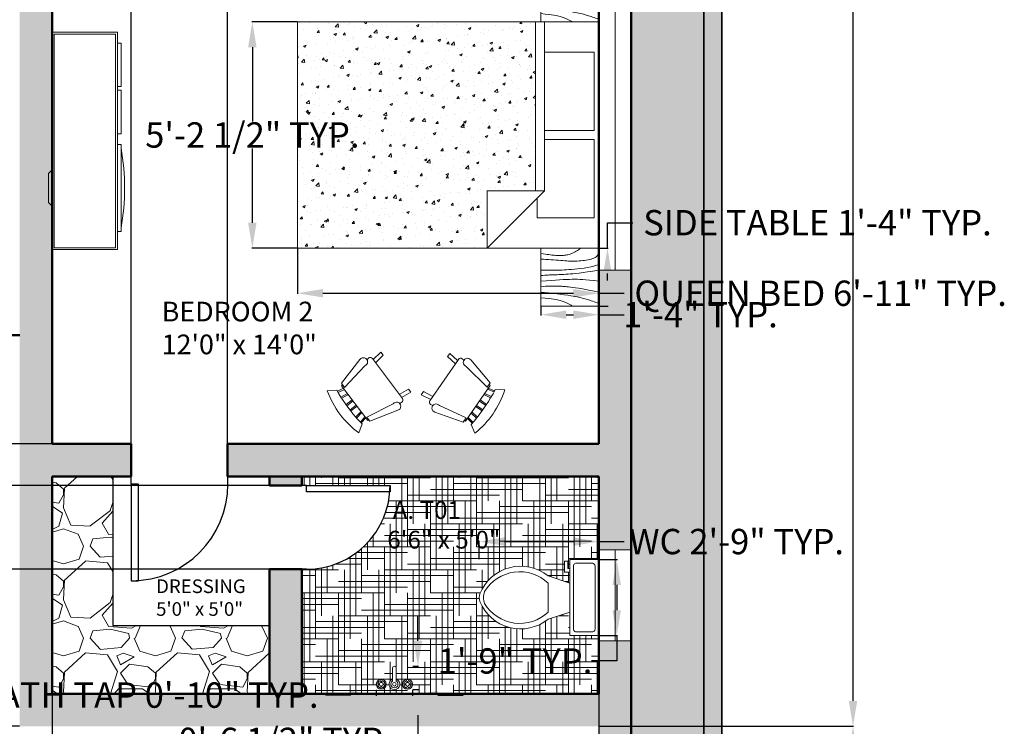
# Model space of a CAD drawing. Units: inches. Extents: x 319 to 870, y 210 to 995.
# Tile 3 of 6: x 598 to 870, y 408 to 603. Entities that reach past the tile are written whole.
import ezdxf

# ---------------------------------------------------------------- set-up
doc = ezdxf.new("R2010")
doc.units = ezdxf.units.IN
doc.header["$MEASUREMENT"] = 0
for name, color, linetype, lineweight in [('A-ANNO-DIMS', 2, 'Continuous', 18), ('A-AREA-IDEN', 7, 'Continuous', 18), ('A-DOOR', 4, 'Continuous', 25), ('A-FLOR-CASE', 7, 'Continuous', 25), ('A-FLOR-CASE-PATT', 252, 'Continuous', 13), ('A-FLOR-FIXT', 9, 'Continuous', 18), ('A-FLOR-PATT', 252, 'Continuous', 13), ('A-FURN', 8, 'Continuous', 18), ('A-GLAZ', 4, 'Continuous', 18), ('A-WALL', 7, 'Continuous', 50), ('A-WALL-PATT', 8, 'Continuous', 13), ('C-PROP', 7, 'Continuous', 35), ('C-PROP-PATT', 8, 'Continuous', 13)]:
    doc.layers.add(name, color=color, linetype=linetype, lineweight=lineweight)
doc.layers.add('A-FURN-PATT', color=30, linetype='Continuous', lineweight=13, true_color=0xf7941d)
doc.layers.add('C-SITE-PATT', color=126, linetype='Continuous', lineweight=13, true_color=0x1e6f63)
doc.styles.get("Standard").update_dxf_attribs({"font": 'arial.ttf'})
doc.dimstyles.get("Standard").update_dxf_attribs({"dimtxt": 7, "dimasz": 7, "dimexe": 0.18, "dimexo": 0.0625, "dimgap": 0.09, "dimtad": 0, "dimtih": 1, "dimtoh": 1, "dimdec": 0, "dimzin": 0, "dimdsep": 46, "dimlunit": 3, "dimtxsty": 'Standard', "dimcen": 0.09, "dimadec": 0, "dimazin": 0, "dimtfac": 1, "dimtdec": 0, "dimtofl": 0, "dimtmove": 0, "dimatfit": 3, "dimfxl": 1, "dimtolj": 1, "dimtzin": 0, "dimarcsym": 0})

# ---------------------------------------------------------------- blocks, each defined once
blk = doc.blocks.new('*U17')
for p, q in [((0, 0), (0, 6)), ((24, 0), (24, 6))]:
    blk.add_line(p, q)
blk.add_lwpolyline([(0, 0), (0, -24), (1.75, -24), (1.75, 0)], close=True)
blk.add_arc((0, 0), 24, 270, 0)
blk = doc.blocks.new('Bed - Queen')
for p, q in [((0, -80.00003), (0, 0)), ((0, 0), (59.99999, 0)), ((59.99999, 0), (59.99999, -80.00003)), ((7.99999, -1.2), (28.79998, -1.2)), ((7.99999, -14.4), (7.99999, -1.2)), ((28.79998, -1.2), (28.79998, -14.4)), ((31.19999, -1.2), (51.99999, -1.2)), ((31.19999, -14.4), (31.19999, -1.2)), ((51.99999, -1.2), (51.99999, -16.4)), ((0, -14.4), (44.8, -14.4)), ((59.99999, -29.6), (44.8, -14.4)), ((44.8, -14.4), (44.8, -29.6)), ((44.8, -16.8), (0, -16.8)), ((51.99999, -16.4), (46.79936, -16.4)), ((44.8, -29.6), (59.99999, -29.6)), ((59.99999, -80.00003), (0, -80.00003))]:
    blk.add_line(p, q)
blk = doc.blocks.new('Entertainment Center')
for p, q in [((-4, 0), (-5, -1)), ((4, 0), (-4, 0)), ((5, -1), (4, 0)), ((-17, -19), (-17, -1)), ((-17, -1), (43, -1)), ((-16.5, -18.5), (-16.5, -1.5)), ((-16.5, -1.5), (42.5, -1.5)), ((42.5, -1.5), (42.5, -18.5)), ((43, -1), (43, -19)), ((43, -19), (-17, -19)), ((42.5, -18.5), (-16.5, -18.5)), ((-12, -20), (-12, -19)), ((12, -19), (12, -20)), ((15, -20), (15, -19)), ((27, -19), (27, -20)), ((28, -20), (28, -19)), ((40, -19), (40, -20)), ((12, -20), (-12, -20)), ((27, -20), (15, -20)), ((40, -20), (28, -20))]:
    blk.add_line(p, q)
blk.add_arc((0, 40), 61, 259.6111, 280.3889)
blk = doc.blocks.new('Toilet - top')
for p, q in [((9.5, -6), (9.5, -2)), ((-8, -8.5), (-8, -8)), ((-7, -8), (-7, -9.5)), ((-4, -8), (-6, -14)), ((4, -8), (6, -14)), ((-10, -8.5), (-8, -8.5)), ((-10, -9.5), (-10, -8.5)), ((-7, -9.5), (-10, -9.5)), ((4, -14), (-4, -14))]:
    blk.add_line(p, q)
blk.add_lwpolyline([(10.5, -8), (10.5, 0), (-10.5, 0), (-10.5, -8)], close=True)
for points in [[(-9.5, -2), (-9.5, -6)], [(8.5, -1), (-8.5, -1)], [(-8.5, -7), (8.5, -7)]]:
    blk.add_lwpolyline(points)
for centre, radius, start, end in [((-8.62, -1.88), 0.884, 81.8699, 188.1301), ((8.62, -1.88), 0.884, 351.8699, 98.1301), ((-8.62, -6.12), 0.884, 171.8699, 278.1301), ((8.62, -6.12), 0.884, 261.8699, 8.1301), ((3.52, -21.58), 12.17, 141.4691, 247.9714), ((4.2, -21.82), 11.33, 136.3677, 238.9468), ((-3.52, -21.58), 12.17, 292.0284, 38.5307), ((-4.2, -21.82), 11.33, 301.053, 43.6321), ((0, -27.88), 4, 245.7318, 294.2682), ((0, -29), 4, 254.8605, 285.1395)]:
    blk.add_arc(centre, radius, start, end)
blk = doc.blocks.new('Chair - Rocking')
for p, q in [((-8, -4.5), (-10, -1.5)), ((8, -4.5), (10, -1.5)), ((-8.23428, -6.99939), (-8.3093, -7.47958)), ((-8.23041, -7), (8.23915, -7)), ((-7.5, -4.5), (-7, -7)), ((-6.5, -7), (-7.02225, -4.43)), ((-4.5, -7), (-4.96674, -4.19951)), ((-4, -7), (-4.40532, -4.16272)), ((-1.5, -4.05012), (-1.5, -7)), ((-1, -7), (-1, -4.05012)), ((1, -7), (1, -4.04655)), ((1.5, -4.05012), (1.5, -7)), ((4, -7), (4.40187, -4.18694)), ((4.5, -7), (4.96761, -4.19437)), ((6.5, -7), (7, -4.4057)), ((7.5, -4.5), (7, -7)), ((8.31071, -7.48854), (8.23449, -7.00073)), ((-9, -7.5), (-12, -18.49999)), ((-7, -7.5), (-9, -7.5)), ((-9, -18.49999), (-7, -7.5)), ((7, -7.5), (9, -7.5)), ((9, -18.49999), (7, -7.5)), ((9, -7.5), (12, -18.49999)), ((-10.36644, -20.64523), (-10.5, -21.49999)), ((10.5, -21.49999), (10.3575, -20.58798)), ((-9, -22.49999), (-9.5, -26.49999)), ((0, -22.49999), (-9.5, -22.49999)), ((-8, -26.49999), (-7.5, -22.49999)), ((0, -22.49999), (9.5, -22.49999)), ((8, -26.49999), (7.5, -22.49999)), ((9, -22.49999), (9.5, -26.49999)), ((-9.5, -26.49999), (-8, -26.49999)), ((9.5, -26.49999), (8, -26.49999))]:
    blk.add_line(p, q)
for centre, radius, start, end in [((0, -34.08333), 34.08333, 72.93847, 107.0615), ((0, -68.25004), 64.25, 93.92211, 97.15267), ((0, -68.25004), 64.25, 82.84733, 93.92211), ((-10.5, -18.99999), 1.58114, 161.5651, 18.43495), ((10.5, -18.99999), 1.58114, 161.5651, 18.43495), ((-9.5, -21.49999), 1, 180, 270), ((9.5, -21.49999), 1, 270, 0)]:
    blk.add_arc(centre, radius, start, end)
blk = doc.blocks.new('Faucet - Bathroom top')
for p, q in [((-4.107, 0.125), (-4.375, 0.125)), ((-3.75, 0.4788), (-3.75, 0.75)), ((-3.5, 0.482), (-3.5, 0.75)), ((-3.1461, 0.125), (-2.875, 0.125)), ((3.143, 0.125), (2.875, 0.125)), ((3.5, 0.4788), (3.5, 0.75)), ((3.75, 0.482), (3.75, 0.75)), ((4.1039, 0.125), (4.375, 0.125)), ((-4.1039, -0.125), (-4.375, -0.125)), ((-3.75, -0.4821), (-3.75, -0.75)), ((-3.5, -0.4789), (-3.5, -0.75)), ((-3.143, -0.125), (-2.875, -0.125)), ((-0.5, -0.8639), (-0.5, -4.5)), ((0.5, -4.5), (0.5, -0.8631)), ((3.1461, -0.125), (2.875, -0.125)), ((3.5, -0.4821), (3.5, -0.75)), ((3.75, -0.4789), (3.75, -0.75)), ((4.107, -0.125), (4.375, -0.125))]:
    blk.add_line(p, q)
for centre, radius in [((-3.625, 0), 1.375), ((-4.625, 0), 0.2795), ((-3.625, 0), 0.5), ((-3.625, 1), 0.2795), ((-2.625, 0), 0.2795), ((0, 0), 0.5), ((3.625, 0), 1.375), ((2.625, 0), 0.2795), ((3.625, 0), 0.5), ((3.625, 1), 0.2795), ((4.625, 0), 0.2795), ((-3.625, -1), 0.2795), ((3.625, -1), 0.2795)]:
    blk.add_circle(centre, radius)
for centre, radius, start, end in [((-3.625, 0), 1, 105.2407, 164.2093), ((-3.625, 0), 1, 16.44125, 74.07887), ((0, 0), 1.5, 289.6514, 250.3603), ((0, 0), 1, 300.3431, 239.7554), ((3.625, 0), 1, 106.12, 164.0884), ((3.625, 0), 1, 16.23422, 73.90469), ((-3.625, 0), 1, 196.2342, 253.9047), ((-3.625, 0), 1, 286.12, 344.0884), ((3.625, 0), 1, 196.4413, 254.0789), ((3.625, 0), 1, 285.2407, 344.2093), ((0, -4.5), 0.5, 180, 0)]:
    blk.add_arc(centre, radius, start, end)
blk = doc.blocks.new('Table - Square Woodgrain 42 x 42 in.')
blk.add_line((0, -42), (42, -42))
for points in [[(0, -4), (1.704, -4.2172), (3.2358, -4.4188), (4.615, -4.604), (5.8615, -4.7721), (6.9951, -4.9224), (8.0357, -5.0541), (9.0031, -5.1667), (9.9171, -5.2594), (10.7951, -5.3316), (11.6445, -5.3836), (12.4702, -5.4157), (13.277, -5.4283), (14.0698, -5.4217), (14.8535, -5.3964), (15.6331, -5.3526), (16.4133, -5.2908), (17.1986, -5.2103), (17.9913, -5.1062), (18.793, -4.9727), (19.6056, -4.8038), (20.4307, -4.5937), (21.2701, -4.3365), (22.1256, -4.0262), (22.9989, -3.6571), (23.888, -3.2272), (24.7756, -2.7516), (25.6408, -2.2491), (26.4624, -1.7387), (27.2195, -1.2395), (27.891, -0.7703), (28.456, -0.3501), (28.8934, 0.002)], [(0, -42), (0, 0), (42, 0), (42, -42)], [(0, -8), (1.8203, -8.1001), (3.6741, -8.2149), (5.5411, -8.3408), (7.4011, -8.4741), (9.2339, -8.6112), (11.0193, -8.7484), (12.7371, -8.8821), (14.3671, -9.0086), (15.8954, -9.1246), (17.3337, -9.2278), (18.6997, -9.3159), (20.0116, -9.387), (21.2871, -9.4389), (22.5442, -9.4696), (23.8008, -9.477), (25.0749, -9.459), (26.3791, -9.4137), (27.7049, -9.3403), (29.0383, -9.2382), (30.3655, -9.1068), (31.6728, -8.9455), (32.9461, -8.7535), (34.1717, -8.5304), (35.3358, -8.2756), (36.4268, -7.9863), (37.443, -7.6521), (38.3849, -7.2603), (39.253, -6.7986), (40.048, -6.2542), (40.7705, -5.6147), (41.421, -4.8674), (42, -4)], [(42, -12), (39.1784, -12.8621), (36.4519, -13.5654), (33.8246, -14.1294), (31.3004, -14.5731), (28.8832, -14.9161), (26.577, -15.1775), (24.3858, -15.3768), (22.3136, -15.5332), (20.3622, -15.6632), (18.5254, -15.7718), (16.7947, -15.8612), (15.1618, -15.9338), (13.6183, -15.9916), (12.1558, -16.0369), (10.7659, -16.0718), (9.4403, -16.0987), (8.1703, -16.1191), (6.9461, -16.1325), (5.7577, -16.1377), (4.595, -16.1335), (3.4479, -16.1188), (2.3064, -16.0924), (1.1604, -16.0532), (0, -16)], [(42, -16), (37.6529, -16.7365), (33.8802, -17.329), (30.6179, -17.7961), (27.8015, -18.1561), (25.3668, -18.4275), (23.2497, -18.6288), (21.3859, -18.7785), (19.7111, -18.8949), (18.1693, -18.9939), (16.7375, -19.0795), (15.401, -19.1534), (14.1449, -19.217), (12.9544, -19.2717), (11.8148, -19.3191), (10.7113, -19.3606), (9.6291, -19.3976), (8.5534, -19.4323), (7.47, -19.4689), (6.3643, -19.5122), (5.222, -19.5672), (4.0288, -19.6386), (2.7703, -19.7313), (1.4321, -19.8501), (0, -20)], [(0, -24), (3.9243, -23.6805), (7.4766, -23.4138), (10.6891, -23.1954), (13.5943, -23.0205), (16.2247, -22.8847), (18.6125, -22.7832), (20.7903, -22.7116), (22.7903, -22.6651), (24.6563, -22.642), (26.4764, -22.6507), (28.35, -22.7024), (30.3766, -22.8084), (32.6555, -22.98), (35.2861, -23.2283), (38.3678, -23.5645), (42, -24)], [(42, -32), (37.392, -31.017), (33.4585, -30.2231), (30.1291, -29.5949), (27.3334, -29.109), (25.0009, -28.742), (23.0612, -28.4707), (21.4439, -28.2716), (20.0786, -28.1215), (18.8998, -28.0002), (17.8609, -27.9014), (16.9206, -27.8219), (16.0371, -27.7588), (15.1691, -27.709), (14.2748, -27.6693), (13.3128, -27.6368), (12.2415, -27.6083), (11.0295, -27.5824), (9.6867, -27.5643), (8.233, -27.5608), (6.6884, -27.5787), (5.0728, -27.6248), (3.4062, -27.7058), (1.7086, -27.8286), (0, -28)], [(0, -32), (5.4026, -32.5358), (9.9494, -33.019), (13.7424, -33.4553), (16.8834, -33.8505), (19.4743, -34.2106), (21.6171, -34.5413), (23.4136, -34.8486), (24.9657, -35.1382), (26.3614, -35.4156), (27.6332, -35.6841), (28.7995, -35.9467), (29.8788, -36.2064), (30.8897, -36.4661), (31.8507, -36.7288), (32.7802, -36.9973), (33.6968, -37.2747), (34.6175, -37.5635), (35.5531, -37.8651), (36.5128, -38.1805), (37.506, -38.5108), (38.5421, -38.8568), (39.6302, -39.2197), (40.7797, -39.6004), (42, -40)], [(0, -36), (3.0098, -36.2857), (5.5354, -36.5643), (7.6368, -36.8359), (9.374, -37.1009), (10.807, -37.3597), (11.9957, -37.6126), (13.0002, -37.8599), (13.8804, -38.102), (14.6874, -38.3393), (15.4365, -38.5729), (16.1338, -38.8041), (16.7858, -39.0341), (17.3987, -39.264), (17.9787, -39.4952), (18.5322, -39.7288), (19.0655, -39.9662), (19.5832, -40.2081), (20.0842, -40.4544), (20.5657, -40.7046), (21.0249, -40.9581), (21.459, -41.2144), (21.8653, -41.4731), (22.2409, -41.7335), (22.5831, -41.9951)]]:
    blk.add_lwpolyline(points)
blk = doc.blocks.new('*U19')
for p, q in [((0, 0), (0, -6)), ((24, 0), (24, -6))]:
    blk.add_line(p, q)
blk.add_lwpolyline([(0, 0), (0, 24), (1.75, 24), (1.75, 0)], close=True)
blk.add_arc((0, 0), 24, 0, 90)
blk = doc.blocks.new('*D27')
at = {"layer": 'A-ANNO-DIMS', "color": 0, "lineweight": -2, "transparency": 16777216}
for p, q in [((760.08, 539.7), (760.08, 546.7)), ((760.08, 546.7), (767.08, 546.7)), ((757.75, 539.7), (760.26, 539.7)), ((760.08, 530.7), (760.08, 532.7)), ((757.75, 523.7), (760.26, 523.7))]:
    blk.add_line(p, q, dxfattribs=at)
at = {"layer": 'A-ANNO-DIMS', "color": 0, "transparency": 16777216}
for points in [[(758.92, 532.7), (761.25, 532.7), (760.08, 539.7)], [(758.92, 530.7), (761.25, 530.7), (760.08, 523.7)]]:
    blk.add_solid(points, dxfattribs=at)
at = {"layer": 'Defpoints', "color": 0, "transparency": 16777216}
for p in [(757.68, 539.7), (760.08, 539.7), (757.68, 523.7)]:
    blk.add_point(p, dxfattribs=at)
at = {"layer": 'A-ANNO-DIMS', "color": 0, "transparency": 16777216, "insert": (818.11, 546.7), "char_height": 7, "attachment_point": 5}
blk.add_mtext('\\A1;SIDE TABLE 1\'-4" TYP.', dxfattribs=at)
blk = doc.blocks.new('*D28')
at = {"layer": 'A-ANNO-DIMS', "color": 0, "lineweight": -2, "transparency": 16777216}
for p, q in [((741.69, 523.64), (741.69, 521.12)), ((757.68, 523.64), (757.68, 521.12)), ((748.69, 521.3), (750.68, 521.3)), ((757.68, 521.3), (764.68, 521.3))]:
    blk.add_line(p, q, dxfattribs=at)
at = {"layer": 'A-ANNO-DIMS', "color": 0, "transparency": 16777216}
for points in [[(748.69, 522.47), (748.69, 520.14), (741.69, 521.3)], [(750.68, 522.47), (750.68, 520.14), (757.68, 521.3)]]:
    blk.add_solid(points, dxfattribs=at)
at = {"layer": 'Defpoints', "color": 0, "transparency": 16777216}
for p in [(741.69, 523.7), (757.68, 523.7), (757.68, 521.3)]:
    blk.add_point(p, dxfattribs=at)
at = {"layer": 'A-ANNO-DIMS', "color": 0, "transparency": 16777216, "insert": (785.78, 521.3), "char_height": 7, "attachment_point": 5}
blk.add_mtext('\\A1;1\'-4" TYP.', dxfattribs=at)
blk = doc.blocks.new('*D31')
at = {"layer": 'A-ANNO-DIMS', "color": 0, "lineweight": -2, "transparency": 16777216}
for p, q in [((674.45, 539.64), (674.45, 527.04)), ((757.68, 539.64), (757.68, 527.04)), ((681.45, 527.22), (750.68, 527.22)), ((757.68, 527.22), (764.68, 527.22))]:
    blk.add_line(p, q, dxfattribs=at)
at = {"layer": 'A-ANNO-DIMS', "color": 0, "transparency": 16777216}
for points in [[(681.45, 528.39), (681.45, 526.05), (674.45, 527.22)], [(750.68, 528.39), (750.68, 526.05), (757.68, 527.22)]]:
    blk.add_solid(points, dxfattribs=at)
at = {"layer": 'Defpoints', "color": 0, "transparency": 16777216}
for p in [(674.45, 539.7), (757.68, 539.7), (757.68, 527.22)]:
    blk.add_point(p, dxfattribs=at)
at = {"layer": 'A-ANNO-DIMS', "color": 0, "transparency": 16777216, "insert": (818.98, 527.22), "char_height": 7, "attachment_point": 5}
blk.add_mtext('\\A1;QUEEN BED 6\'-11" TYP.', dxfattribs=at)
blk = doc.blocks.new('*D32')
at = {"layer": 'A-ANNO-DIMS', "color": 0, "lineweight": -2, "transparency": 16777216}
for p, q in [((674.39, 602.13), (661.79, 602.13)), ((661.97, 595.13), (661.97, 574.63)), ((661.97, 546.7), (661.97, 567.21)), ((674.39, 539.7), (661.79, 539.7))]:
    blk.add_line(p, q, dxfattribs=at)
at = {"layer": 'A-ANNO-DIMS', "color": 0, "transparency": 16777216}
for points in [[(660.8, 595.13), (663.13, 595.13), (661.97, 602.13)], [(660.8, 546.7), (663.13, 546.7), (661.97, 539.7)]]:
    blk.add_solid(points, dxfattribs=at)
at = {"layer": 'Defpoints', "color": 0, "transparency": 16777216}
for p in [(674.45, 602.13), (661.97, 539.7), (674.45, 539.7)]:
    blk.add_point(p, dxfattribs=at)
at = {"layer": 'A-ANNO-DIMS', "color": 0, "transparency": 16777216, "insert": (661.97, 570.92), "char_height": 7, "attachment_point": 5}
blk.add_mtext('\\A1;5\'-2 1/2" TYP.', dxfattribs=at)
blk = doc.blocks.new('*D35')
at = {"layer": 'A-ANNO-DIMS', "color": 0, "lineweight": -2, "transparency": 16777216}
for p, q in [((654.78, 626.45), (654.78, 610.9)), ((757.68, 626.45), (757.68, 610.9)), ((661.78, 611.08), (666.54, 611.08)), ((750.68, 611.08), (745.92, 611.08))]:
    blk.add_line(p, q, dxfattribs=at)
at = {"layer": 'A-ANNO-DIMS', "color": 0, "transparency": 16777216}
for points in [[(661.78, 612.24), (661.78, 609.91), (654.78, 611.08)], [(750.68, 612.24), (750.68, 609.91), (757.68, 611.08)]]:
    blk.add_solid(points, dxfattribs=at)
at = {"layer": 'Defpoints', "color": 0, "transparency": 16777216}
for p in [(654.78, 626.51), (757.68, 626.51), (757.68, 611.08)]:
    blk.add_point(p, dxfattribs=at)
at = {"layer": 'A-ANNO-DIMS', "color": 0, "transparency": 16777216, "insert": (706.23, 611.08), "char_height": 7, "attachment_point": 5}
blk.add_mtext('\\A1;WARDROBE 8\'-7"', dxfattribs=at)
blk = doc.blocks.new('*D37')
at = {"layer": 'A-ANNO-DIMS', "color": 0, "lineweight": -2, "transparency": 16777216}
for p, q in [((724.64, 453.77), (724.64, 458.85)), ((731.64, 458.67), (750.68, 458.67)), ((757.68, 453.77), (757.68, 458.85)), ((757.68, 458.67), (764.68, 458.67))]:
    blk.add_line(p, q, dxfattribs=at)
at = {"layer": 'A-ANNO-DIMS', "color": 0, "transparency": 16777216}
for points in [[(731.64, 459.83), (731.64, 457.5), (724.64, 458.67)], [(750.68, 459.83), (750.68, 457.5), (757.68, 458.67)]]:
    blk.add_solid(points, dxfattribs=at)
at = {"layer": 'Defpoints', "color": 0, "transparency": 16777216}
for p in [(757.68, 458.67), (724.64, 453.71), (757.68, 453.71)]:
    blk.add_point(p, dxfattribs=at)
at = {"layer": 'A-ANNO-DIMS', "color": 0, "transparency": 16777216, "insert": (795.76, 458.67), "char_height": 7, "attachment_point": 5}
blk.add_mtext('\\A1;WC 2\'-9" TYP.', dxfattribs=at)
blk = doc.blocks.new('*D38')
at = {"layer": 'A-ANNO-DIMS', "color": 0, "lineweight": -2, "transparency": 16777216}
for p, q in [((757.75, 453.71), (762.82, 453.71)), ((762.64, 446.71), (762.64, 439.71)), ((757.75, 432.71), (762.82, 432.71)), ((762.64, 432.71), (762.64, 425.71)), ((762.64, 425.71), (755.64, 425.71))]:
    blk.add_line(p, q, dxfattribs=at)
at = {"layer": 'A-ANNO-DIMS', "color": 0, "transparency": 16777216}
for points in [[(761.48, 446.71), (763.81, 446.71), (762.64, 453.71)], [(761.48, 439.71), (763.81, 439.71), (762.64, 432.71)]]:
    blk.add_solid(points, dxfattribs=at)
at = {"layer": 'Defpoints', "color": 0, "transparency": 16777216}
for p in [(757.68, 453.71), (757.68, 432.71), (762.64, 432.71)]:
    blk.add_point(p, dxfattribs=at)
at = {"layer": 'A-ANNO-DIMS', "color": 0, "transparency": 16777216, "insert": (734.55, 425.71), "char_height": 7, "attachment_point": 5}
blk.add_mtext('\\A1;1\'-9" TYP.', dxfattribs=at)
blk = doc.blocks.new('*D39')
at = {"layer": 'A-ANNO-DIMS', "color": 0, "lineweight": -2, "transparency": 16777216}
for p, q in [((689.21, 416.28), (682.21, 416.28)), ((696.21, 417.72), (696.21, 416.1)), ((706.21, 417.72), (706.21, 416.1)), ((713.21, 416.28), (720.21, 416.28))]:
    blk.add_line(p, q, dxfattribs=at)
at = {"layer": 'A-ANNO-DIMS', "color": 0, "transparency": 16777216}
for points in [[(689.21, 417.45), (689.21, 415.11), (696.21, 416.28)], [(713.21, 417.45), (713.21, 415.11), (706.21, 416.28)]]:
    blk.add_solid(points, dxfattribs=at)
at = {"layer": 'Defpoints', "color": 0, "transparency": 16777216}
for p in [(696.21, 417.78), (696.21, 416.28), (706.21, 417.78)]:
    blk.add_point(p, dxfattribs=at)
at = {"layer": 'A-ANNO-DIMS', "color": 0, "transparency": 16777216, "insert": (632.95, 416.28), "char_height": 7, "attachment_point": 5}
blk.add_mtext('\\A1;BATH TAP 0\'-10" TYP.', dxfattribs=at)
blk = doc.blocks.new('*D40')
at = {"layer": 'A-ANNO-DIMS', "color": 0, "lineweight": -2, "transparency": 16777216}
for p, q in [((707.71, 431.28), (707.71, 438.28)), ((706.27, 424.28), (707.89, 424.28)), ((706.27, 417.78), (707.89, 417.78)), ((707.71, 410.78), (707.71, 403.78)), ((707.71, 403.78), (700.71, 403.78))]:
    blk.add_line(p, q, dxfattribs=at)
at = {"layer": 'A-ANNO-DIMS', "color": 0, "transparency": 16777216}
for points in [[(706.54, 431.28), (708.87, 431.28), (707.71, 424.28)], [(706.54, 410.78), (708.87, 410.78), (707.71, 417.78)]]:
    blk.add_solid(points, dxfattribs=at)
at = {"layer": 'Defpoints', "color": 0, "transparency": 16777216}
for p in [(706.21, 424.28), (706.21, 417.78), (707.71, 417.78)]:
    blk.add_point(p, dxfattribs=at)
at = {"layer": 'A-ANNO-DIMS', "color": 0, "transparency": 16777216, "insert": (671.13, 403.78), "char_height": 7, "attachment_point": 5}
blk.add_mtext('\\A1;0\'-6 1/2" TYP.', dxfattribs=at)
blk = doc.blocks.new('*D50')
at = {"layer": 'A-ANNO-DIMS', "color": 0, "lineweight": -2, "transparency": 16777216}
for p, q in [((766.75, 923.67), (828.11, 923.67)), ((827.93, 916.67), (827.93, 669.33)), ((827.93, 414.67), (827.93, 662)), ((757.75, 407.67), (828.11, 407.67))]:
    blk.add_line(p, q, dxfattribs=at)
at = {"layer": 'A-ANNO-DIMS', "color": 0, "transparency": 16777216}
for points in [[(826.77, 916.67), (829.1, 916.67), (827.93, 923.67)], [(826.77, 414.67), (829.1, 414.67), (827.93, 407.67)]]:
    blk.add_solid(points, dxfattribs=at)
at = {"layer": 'Defpoints', "color": 0, "transparency": 16777216}
for p in [(766.68, 923.67), (827.93, 923.67), (757.68, 407.67)]:
    blk.add_point(p, dxfattribs=at)
at = {"layer": 'A-ANNO-DIMS', "color": 0, "transparency": 16777216, "insert": (827.93, 665.67), "char_height": 7, "attachment_point": 5}
blk.add_mtext('\\A1;43\'-0"', dxfattribs=at)
blk = doc.blocks.new('*D51')
at = {"layer": 'A-ANNO-DIMS', "color": 0, "lineweight": -2, "transparency": 16777216}
for p, q in [((757.75, 407.67), (828.11, 407.67)), ((827.93, 400.67), (827.93, 369.83)), ((827.93, 331.67), (827.93, 362.5)), ((791.75, 324.67), (828.11, 324.67))]:
    blk.add_line(p, q, dxfattribs=at)
at = {"layer": 'A-ANNO-DIMS', "color": 0, "transparency": 16777216}
for points in [[(826.77, 400.67), (829.1, 400.67), (827.93, 407.67)], [(826.77, 331.67), (829.1, 331.67), (827.93, 324.67)]]:
    blk.add_solid(points, dxfattribs=at)
at = {"layer": 'Defpoints', "color": 0, "transparency": 16777216}
for p in [(757.68, 407.67), (827.93, 407.67), (791.68, 324.67)]:
    blk.add_point(p, dxfattribs=at)
at = {"layer": 'A-ANNO-DIMS', "color": 0, "transparency": 16777216, "insert": (827.93, 366.17), "char_height": 7, "attachment_point": 5}
blk.add_mtext('\\A1;6\'-11"', dxfattribs=at)
blk = doc.blocks.new('*D53')
at = {"layer": 'A-ANNO-DIMS', "color": 0, "lineweight": -2, "transparency": 16777216}
for p, q in [((606.68, 416.61), (606.68, 214.45)), ((757.68, 416.61), (757.68, 214.45)), ((613.68, 214.63), (670.4, 214.63)), ((750.68, 214.63), (693.97, 214.63))]:
    blk.add_line(p, q, dxfattribs=at)
at = {"layer": 'A-ANNO-DIMS', "color": 0, "transparency": 16777216}
for points in [[(613.68, 215.8), (613.68, 213.47), (606.68, 214.63)], [(750.68, 215.8), (750.68, 213.47), (757.68, 214.63)]]:
    blk.add_solid(points, dxfattribs=at)
at = {"layer": 'Defpoints', "color": 0, "transparency": 16777216}
for p in [(606.68, 416.67), (757.68, 416.67), (757.68, 214.63)]:
    blk.add_point(p, dxfattribs=at)
at = {"layer": 'A-ANNO-DIMS', "color": 0, "transparency": 16777216, "insert": (682.18, 214.63), "char_height": 7, "attachment_point": 5}
blk.add_mtext('\\A1;12\'-7"', dxfattribs=at)
blk = doc.blocks.new('*D54')
at = {"layer": 'A-ANNO-DIMS', "color": 0, "lineweight": -2, "transparency": 16777216}
for p, q in [((606.62, 485.67), (334.2, 485.67)), ((334.38, 478.67), (334.38, 450.33)), ((334.38, 414.67), (334.38, 443)), ((597.62, 407.67), (334.2, 407.67))]:
    blk.add_line(p, q, dxfattribs=at)
at = {"layer": 'A-ANNO-DIMS', "color": 0, "transparency": 16777216}
for points in [[(333.21, 478.67), (335.55, 478.67), (334.38, 485.67)], [(333.21, 414.67), (335.55, 414.67), (334.38, 407.67)]]:
    blk.add_solid(points, dxfattribs=at)
at = {"layer": 'Defpoints', "color": 0, "transparency": 16777216}
for p in [(334.38, 485.67), (606.68, 485.67), (597.68, 407.67)]:
    blk.add_point(p, dxfattribs=at)
at = {"layer": 'A-ANNO-DIMS', "color": 0, "transparency": 16777216, "insert": (334.38, 446.67), "char_height": 7, "attachment_point": 5}
blk.add_mtext('\\A1;6\'-6"', dxfattribs=at)
blk = doc.blocks.new('*D55')
at = {"layer": 'A-ANNO-DIMS', "color": 0, "lineweight": -2, "transparency": 16777216}
for p, q in [((628.53, 485.73), (628.53, 985.1)), ((635.53, 984.92), (648.14, 984.92)), ((655.14, 485.73), (655.14, 985.1)), ((655.14, 984.92), (662.14, 984.92))]:
    blk.add_line(p, q, dxfattribs=at)
at = {"layer": 'A-ANNO-DIMS', "color": 0, "transparency": 16777216}
for points in [[(635.53, 986.09), (635.53, 983.75), (628.53, 984.92)], [(648.14, 986.09), (648.14, 983.75), (655.14, 984.92)]]:
    blk.add_solid(points, dxfattribs=at)
at = {"layer": 'Defpoints', "color": 0, "transparency": 16777216}
for p in [(655.14, 984.92), (628.53, 485.67), (655.14, 485.67)]:
    blk.add_point(p, dxfattribs=at)
at = {"layer": 'A-ANNO-DIMS', "color": 0, "transparency": 16777216, "insert": (679.75, 984.92), "char_height": 7, "attachment_point": 5}
blk.add_mtext('\\A1;2\'-2 1/2"', dxfattribs=at)
blk = doc.blocks.new('*D56')
at = {"layer": 'A-ANNO-DIMS', "color": 0, "lineweight": -2, "transparency": 16777216}
for p, q in [((675.62, 474.1), (334.2, 474.1)), ((334.38, 467.1), (334.38, 466.2)), ((334.38, 458.09), (334.38, 458.99)), ((675.62, 451.09), (334.2, 451.09))]:
    blk.add_line(p, q, dxfattribs=at)
at = {"layer": 'A-ANNO-DIMS', "color": 0, "transparency": 16777216}
for points in [[(333.21, 467.1), (335.55, 467.1), (334.38, 474.1)], [(333.21, 458.09), (335.55, 458.09), (334.38, 451.09)]]:
    blk.add_solid(points, dxfattribs=at)
at = {"layer": 'Defpoints', "color": 0, "transparency": 16777216}
for p in [(334.38, 474.1), (675.68, 474.1), (675.68, 451.09)]:
    blk.add_point(p, dxfattribs=at)
at = {"layer": 'A-ANNO-DIMS', "color": 0, "transparency": 16777216, "insert": (334.38, 462.6), "char_height": 7, "attachment_point": 5}
blk.add_mtext('\\A1;1\'-11"', dxfattribs=at)

msp = doc.modelspace()

# ---------------------------------------------------------------- hatches: boundary and pattern name
at = {"layer": 'A-FLOR-CASE-PATT'}
h = msp.add_hatch(dxfattribs=at)
h.set_pattern_fill('GRAVEL', color=256)
h.set_pattern_definition([(228.0128, (18.288, 25.4), (-203.2, -228.6), [3.4172, -338.30484]), (184.96974, (16.002, 22.86), (304.7999999, 25.4000014), [5.86405, -580.5405]), (132.51045, (10.16, 22.352), (254, -279.4), [4.1348, -409.34723]), (267.27369, (0.254, 16.002), (25.4, 508), [5.34005, -528.66437]), (292.83365, (0, 10.668), (-127, 304.8), [5.23634, -518.3981]), (357.27369, (2.032, 5.842), (-508, 25.4), [5.34005, -528.66437]), (37.69424, (7.366, 5.588), (-330.2, -254), [7.06194, -699.13115]), (72.25533, (12.954, 9.906), (177.8, 558.8), [6.6672, -660.05257]), (121.42957, (14.986, 16.256), (-203.2, 330.2), [5.35813, -530.45546]), (175.23636, (12.192, 20.828), (279.4, -25.4), [6.11713, -299.73937]), (222.39744, (6.096, 21.336), (-304.8, -279.4), [7.91078, -783.16773]), (138.81407, (25.4, 15.748), (-177.8, 152.4), [2.70005, -267.30566]), (171.46923, (23.368, 17.526), (330.2, -50.8), [5.1368, -508.5464]), (225, (18.288, 18.288), (-4e-15, -25.4), [3.5921, -32.3289]), (203.1986, (16.51, 21.336), (127, 50.8), [1.9344, -191.5062]), (291.8014, (14.732, 20.574), (-25.4, 76.2), [2.73566, -134.0475]), (30.96376, (15.748, 18.034), (76.2, 50.8), [4.4432, -143.663]), (161.565, (19.558, 20.32), (50.8, -25.4), [3.2129, -77.109]), (16.38954, (0, 20.574), (254, 76.2), [4.5009, -445.58827]), (70.34618, (4.318, 21.844), (-101.6, -279.4), [3.776, -373.82216]), (293.1986, (19.558, 25.4), (-50.8, 127), [3.8688, -189.57184]), (343.61046, (21.082, 21.844), (-254, 76.2), [4.5009, -445.58827]), (339.44395, (0, 4.826), (-127, 50.8), [4.34035, -212.67734]), (294.77514, (4.064, 3.302), (-127, 279.4), [3.6367, -360.03593]), (66.8014, (19.812, 0), (50.8, 127), [3.8688, -189.57184]), (17.35402, (21.336, 3.556), (-330.2, -101.6), [4.25783, -421.52376]), (69.44395, (7.366, 0), (-50.8, -127), [2.1702, -214.8475]), (101.3099, (18.288, 0), (-25.4, 101.6), [1.29515, -128.21995]), (165.9638, (18.034, 1.27), (76.2, -25.4), [5.23634, -99.49055]), (186.009, (12.954, 2.54), (254, 25.4), [4.85267, -480.41365]), (303.6901, (15.748, 15.748), (-25.4, 50.8), [3.66324, -87.91776]), (353.15723, (17.78, 12.7), (431.8, -50.8), [6.39557, -633.1601]), (60.9454, (24.13, 11.938), (-101.6, -177.8), [2.6151, -258.8939]), (90, (25.4, 14.224), (-25.4, 25.4), [1.524, -23.876]), (120.25644, (12.446, 3.302), (101.6, -177.8), [3.52867, -349.3394]), (48.0128, (10.668, 6.35), (203.2, 228.6), [6.83443, -334.8876]), (0, (15.24, 11.43), (25.4, 25.4), [6.604, -18.796]), (325.30485, (21.844, 11.43), (254, -177.8), [4.0161, -397.59317]), (254.0546, (25.146, 9.144), (-25.4, -101.6), [3.6983, -181.2165]), (207.64598, (24.13, 5.588), (-482.6, -254), [6.02145, -596.12464]), (175.42608, (18.796, 2.794), (-330.2, 25.4), [6.3703, -630.65846])])
h.paths.add_polyline_path([(623.41, 476.67), (606.68, 476.67), (606.68, 416.67), (666.68, 416.67), (666.68, 435.49), (623.41, 435.49)])
at = {"layer": 'A-FLOR-PATT'}
h = msp.add_hatch(dxfattribs=at)
h.set_pattern_fill('HOUND', color=256)
h.set_pattern_definition([(0, (0, 0), (6.35, 1.5875), [25.4, -12.7]), (90, (0, 0), (-1.5875, -6.35), [25.4, -12.7])])
h.paths.add_polyline_path([(757.68, 416.67), (757.68, 432.71), (749.68, 432.71), (749.68, 439.21), (743.69, 437.21, -0.501323), (724.82, 442.16, -0.132891), (724.82, 444.25, -0.501317), (743.68, 449.21), (749.68, 447.21), (749.68, 450.21), (748.18, 450.21), (748.18, 453.21), (749.18, 453.21), (749.18, 451.21), (749.68, 451.21), (749.68, 453.71), (757.68, 453.71), (757.68, 476.67), (675.68, 476.67), (675.68, 474.1), (676.95, 474.1), (700.01, 474.1), (700.01, 472.42), (699.95, 472.42, -0.392996), (676.95, 451.04), (675.68, 451.04), (675.68, 416.67)])
h.paths.add_polyline_path([(701.71, 423.78), (701.71, 420.69, -5.828427), (700.71, 420.69), (700.71, 423.78, -1)], flags=16)
h.paths.add_polyline_path([(706.11, 419.28, -0.455903), (705.79, 419, -0.257992), (705.11, 418.32, -0.61268), (704.83, 417.9, 0.394698)], flags=16)
h.paths.add_polyline_path([(704.96, 420.03), (704.96, 419.76, -0.414214), (705.32, 419.15), (705.31, 419.15), (705.31, 419.42, -1.020482), (704.35, 419.15), (704.08, 419.15, -1.951411), (703.87, 419.56, -0.257992), (704.55, 420.24, -1.951411)], flags=16)
h.paths.add_polyline_path([(701.71, 419.28, -1), (700.71, 419.28, -1)], flags=0)
h.paths.add_polyline_path([(698.86, 419.28, -0.455903), (698.54, 419, -0.257992), (697.86, 418.32, -0.61268), (697.58, 417.9, 0.394698)], flags=16)
h.paths.add_polyline_path([(697.71, 420.03), (697.71, 419.76, -0.414214), (698.07, 419.15), (698.06, 419.15), (698.06, 419.42, -1.020482), (697.1, 419.15), (696.83, 419.15, -1.951411), (696.62, 419.56, -0.257992), (697.3, 420.24, -1.951411)], flags=16)
h.paths.add_polyline_path([(697.76, 454.02), (730.18, 454.02), (730.18, 472.33), (697.76, 472.33)], flags=24)
at = {"layer": 'A-FURN-PATT'}
h = msp.add_hatch(dxfattribs=at)
h.set_pattern_fill('AR-CONC', color=256)
h.set_pattern_definition([(50, (0, 0), (7.172602, -0.62752), [0.75, -8.25]), (355, (0, 0), (-1.387513, 7.52192), [0.6, -6.6]), (100.45144, (0.598, -0.052), (5.78509, 6.8944), [0.6374, -7.01142]), (46.1842, (0, 2), (10.67241, -1.65519), [1.125, -12.375]), (96.6356, (0.889, 1.862), (9.34662, 9.74119), [0.9561, -10.51714]), (351.1842, (0, 2), (9.34662, 9.74119), [0.9, -9.9]), (21, (1, 1.5), (5.96907, -4.02619), [0.75, -8.25]), (326, (1, 1.5), (2.433153, 7.2515), [0.6, -6.6]), (71.45144, (1.4974, 1.1645), (8.402224, 3.22531), [0.6374, -7.01142]), (37.5, (0, 0), (0.1215986, 3.3289385), [0, -6.52, 0, -6.7, 0, -6.625]), (7.5, (0, 0), (2.630695, 3.944117), [0, -3.82, 0, -6.37, 0, -2.525]), (327.5, (-2.23, 0), (5.338224, -0.225549), [0, -2.5, 0, -7.8, 0, -10.35]), (317.5, (-3.23, 0), (5.831862, 1.00105), [0, -3.25, 0, -5.18, 0, -7.35])])
h.paths.add_polyline_path([(726.89, 555.52), (740.21, 555.52), (740.21, 602.13), (674.45, 602.13), (674.45, 539.7), (726.89, 539.7)])
at = {"layer": 'A-WALL-PATT'}
h = msp.add_hatch(color=256, dxfattribs=at)
h.dxf.hatch_style = 1
h.paths.add_polyline_path([(606.68, 476.67), (628.53, 476.67), (628.53, 485.67), (606.68, 485.67), (606.68, 614.99), (597.68, 614.99), (597.68, 407.67), (757.68, 407.67), (757.68, 385.48), (766.68, 385.48), (766.68, 431.25), (757.68, 431.25), (757.68, 416.67), (606.68, 416.67)])
h = msp.add_hatch(color=256, dxfattribs=at)
h.dxf.hatch_style = 1
h.paths.add_polyline_path([(757.68, 485.67), (655.14, 485.67), (655.14, 476.67), (757.68, 476.67), (757.68, 456.34), (766.68, 456.34), (766.68, 533.56), (757.68, 533.56)])
h = msp.add_hatch(color=256, dxfattribs=at)
h.dxf.hatch_style = 1
h.paths.add_polyline_path([(675.68, 474.1), (675.68, 476.67), (666.68, 476.67), (666.68, 474.1)])
h = msp.add_hatch(color=256, dxfattribs=at)
h.dxf.hatch_style = 1
h.paths.add_polyline_path([(675.68, 451.09), (666.68, 451.09), (666.68, 416.67), (675.68, 416.67)])
at = {"layer": 'C-PROP-PATT'}
h = msp.add_hatch(color=256, dxfattribs=at)
h.dxf.hatch_style = 1
h.paths.add_polyline_path([(757.68, 329.67), (597.68, 329.67), (597.68, 324.67), (791.68, 324.67), (791.68, 948.67), (376.68, 948.67), (376.68, 943.67), (786.68, 943.67), (786.68, 329.67), (766.68, 329.67), (766.68, 354.04), (757.68, 354.04)])
at = {"layer": 'C-SITE-PATT'}
h = msp.add_hatch(color=256, dxfattribs=at)
h.dxf.hatch_style = 1
h.paths.add_polyline_path([(376.68, 515.67), (396.68, 515.67), (396.68, 923.67), (528.68, 923.67), (606.68, 923.67), (766.68, 923.67), (766.68, 329.67), (786.68, 329.67), (786.68, 943.67), (376.68, 943.67)])
h.paths.add_polyline_path([(392.17, 638.98), (392.17, 682.3), (381.61, 682.3), (381.61, 638.98)], flags=24)
h.paths.add_polyline_path([(772.77, 716.95), (772.77, 673.64), (783.33, 673.64), (783.33, 716.95)], flags=24)
h.paths.add_polyline_path([(542.27, 929.56), (581.61, 929.56), (581.61, 939.15), (542.27, 939.15)], flags=24)

# ---------------------------------------------------------------- linework, layer by layer
at = {"layer": 'A-FLOR-CASE'}
for p, q in [((623.41, 476.67), (623.41, 435.49)), ((623.41, 435.49), (666.68, 435.49))]:
    msp.add_line(p, q, dxfattribs=at)
at = {"layer": 'A-GLAZ'}
for p, q in [((762.18, 605.29), (762.18, 533.56)), ((757.68, 533.56), (766.68, 533.56)), ((757.68, 456.34), (766.68, 456.34)), ((762.18, 456.34), (762.18, 431.25)), ((757.68, 431.25), (766.68, 431.25))]:
    msp.add_line(p, q, dxfattribs=at)
at = {"layer": 'A-WALL'}
for p, q in [((766.68, 329.67), (766.68, 923.67)), ((766.68, 731.67), (766.68, 329.67)), ((757.68, 653.67), (757.68, 485.67)), ((606.68, 614.99), (606.68, 485.67)), ((594.44, 515.67), (597.68, 515.67)), ((628.53, 485.67), (606.68, 485.67)), ((628.53, 485.67), (628.53, 476.67)), ((757.68, 485.67), (655.14, 485.67)), ((655.14, 476.67), (655.14, 485.67)), ((606.68, 476.67), (606.68, 416.67)), ((628.53, 476.67), (606.68, 476.67)), ((757.68, 476.67), (655.14, 476.67)), ((666.68, 476.67), (666.68, 474.1)), ((675.68, 476.67), (675.68, 474.1)), ((757.68, 476.67), (757.68, 416.67)), ((757.68, 476.67), (757.68, 416.67)), ((675.68, 474.1), (666.68, 474.1)), ((666.68, 451.09), (675.68, 451.09)), ((666.68, 451.09), (666.68, 416.67)), ((675.68, 451.09), (675.68, 416.67)), ((757.68, 416.67), (606.68, 416.67))]:
    msp.add_line(p, q, dxfattribs=at)
at = {"layer": 'C-PROP'}
for p, q in [((791.68, 324.67), (791.68, 948.67)), ((786.68, 329.67), (786.68, 943.67))]:
    msp.add_line(p, q, dxfattribs=at)

# ---------------------------------------------------------------- block references
at = {"layer": 'A-DOOR', "xscale": 1.111238952142048, "yscale": 1.111238952142048, "zscale": 1.111238952142048}
msp.add_blockref('*U17', (628.53, 474.5), dxfattribs=at)
at = {"layer": 'A-DOOR', "xscale": 0.9609774732916079, "yscale": 0.9609774732916079, "zscale": 0.9609774732916079, "rotation": 270}
msp.add_blockref('*U19', (676.95, 474.1), dxfattribs=at)
at = {"layer": 'A-FLOR-FIXT'}
for name, p, rotation in [('Toilet - top', (757.68, 443.21), 270.0000000000009), ('Faucet - Bathroom top', (701.21, 419.28), 180)]:
    msp.add_blockref(name, p, dxfattribs=dict(at, rotation=rotation))
at = {"layer": 'A-FURN', "xscale": 0.3809342412266087, "yscale": 0.3809342412266087, "zscale": 0.3809342412266087}
for p in [(741.69, 618.13), (741.69, 539.7)]:
    msp.add_blockref('Table - Square Woodgrain 42 x 42 in.', p, dxfattribs=at)
at = {"layer": 'A-FURN'}
for name, p, xscale, yscale, zscale, rotation in [('Bed - Queen', (757.68, 602.13), 1.0404319622762, 1.0404319622762, 1.0404319622762, 270), ('Chair - Rocking', (686.16, 493.83), 0.7291334553679596, 0.7291334553679596, 0.7291334553679596, 126.8698976458433), ('Chair - Rocking', (728.48, 493.96), 0.7291334553679596, 0.7291334553679596, 0.7291334553679596, 235.4636896259277)]:
    msp.add_blockref(name, p, dxfattribs=dict(at, xscale=xscale, yscale=yscale, zscale=zscale, rotation=rotation))
at = {"layer": 'A-FURN', "rotation": 90}
msp.add_blockref('Entertainment Center', (605.68, 556.26), dxfattribs=at)

# ---------------------------------------------------------------- texts
at = {"layer": 'A-AREA-IDEN', "attachment_point": 1}
for s, width, gutter_width, insert, char_height in [('BEDROOM 2\\P12\'0" x 14\'0"', 70.4063, 27.18, (636.93, 524.88), 5.4365), ('\\pxi-3,l4,t4; A. T01\\P6\'6" x 5\'0"', 63.5478, 24.53, (694.33, 469.82), 4.9069), ('DRESSING\\P5\'0" x 5\'0"', 48.8305, 18.85, (635.38, 448.22), 3.7705)]:
    msp.add_mtext_dynamic_manual_height_columns(s, width=width, gutter_width=gutter_width, heights=[0], dxfattribs=dict(at, insert=insert, char_height=char_height))

# ---------------------------------------------------------------- dimensions: what is measured, and where the dimension line sits
at = {"layer": 'A-ANNO-DIMS'}
for base, p1, p2, picture, middle in [((655.14, 984.92), (628.53, 485.67), (655.14, 485.67), '*D55', (679.75, 984.92)), ((757.68, 214.63), (606.68, 416.67), (757.68, 416.67), '*D53', (682.18, 214.63))]:
    dim = msp.add_linear_dim(base=base, p1=p1, p2=p2, dimstyle='Standard', override={"dimdec": 1, "dimlfac": 1, "dimrnd": 0, "dimzin": 1, "dimdsep": 46, "dimlunit": 4, "dimfrac": 2}, dxfattribs=at)
    dim.commit()
    dim.dimension.update_dxf_attribs({"geometry": picture, "text_midpoint": middle})
for base, p1, p2, picture, middle in [((827.93, 923.67), (757.68, 407.67), (766.68, 923.67), '*D50', (827.93, 665.67)), ((334.38, 485.67), (597.68, 407.67), (606.68, 485.67), '*D54', (334.38, 446.67)), ((334.38, 474.1), (675.68, 451.09), (675.68, 474.1), '*D56', (334.38, 462.6)), ((827.93, 407.67), (791.68, 324.67), (757.68, 407.67), '*D51', (827.93, 366.17))]:
    dim = msp.add_linear_dim(base=base, p1=p1, p2=p2, angle=90, dimstyle='Standard', override={"dimdec": 1, "dimlfac": 1, "dimrnd": 0, "dimzin": 1, "dimdsep": 46, "dimlunit": 4, "dimfrac": 2}, dxfattribs=at)
    dim.commit()
    dim.dimension.update_dxf_attribs({"geometry": picture, "text_midpoint": middle})
for base, p1, p2, text, picture, middle in [((757.68, 611.08), (654.78, 626.51), (757.68, 626.51), 'WARDROBE <>', '*D35', (706.23, 611.08)), ((757.68, 527.22), (674.45, 539.7), (757.68, 539.7), 'QUEEN BED <> TYP.', '*D31', (818.98, 527.22)), ((757.68, 521.3), (741.69, 523.7), (757.68, 523.7), '<> TYP.', '*D28', (785.78, 521.3))]:
    dim = msp.add_linear_dim(base=base, p1=p1, p2=p2, text=text, dimstyle='Standard', override={"dimdec": 1, "dimlfac": 1, "dimrnd": 0, "dimzin": 1, "dimdsep": 46, "dimlunit": 4, "dimfrac": 2}, dxfattribs=at)
    dim.commit()
    dim.dimension.update_dxf_attribs({"geometry": picture, "text_midpoint": middle})
for base, p1, p2, angle, text, picture, middle in [((661.97, 539.7), (674.45, 602.13), (674.45, 539.7), 270, '<> TYP.', '*D32', (661.97, 570.92)), ((760.08, 539.7), (757.68, 523.7), (757.68, 539.7), 90, 'SIDE TABLE <> TYP.', '*D27', (818.11, 546.7)), ((757.68, 458.67), (724.64, 453.71), (757.68, 453.71), 0, 'WC <> TYP.', '*D37', (795.76, 458.67)), ((762.64, 432.71), (757.68, 453.71), (757.68, 432.71), 270, '<> TYP.', '*D38', (734.55, 425.71)), ((696.21, 416.28), (706.21, 417.78), (696.21, 417.78), 180, 'BATH TAP <> TYP.', '*D39', (632.95, 416.28)), ((707.71, 417.78), (706.21, 424.28), (706.21, 417.78), 270, '<> TYP.', '*D40', (671.13, 403.78))]:
    dim = msp.add_linear_dim(base=base, p1=p1, p2=p2, angle=angle, text=text, dimstyle='Standard', override={"dimdec": 1, "dimlfac": 1, "dimrnd": 0, "dimzin": 1, "dimdsep": 46, "dimlunit": 4, "dimfrac": 2}, dxfattribs=at)
    dim.commit()
    dim.dimension.update_dxf_attribs({"geometry": picture, "text_midpoint": middle})

doc.saveas('drawing.dxf')
